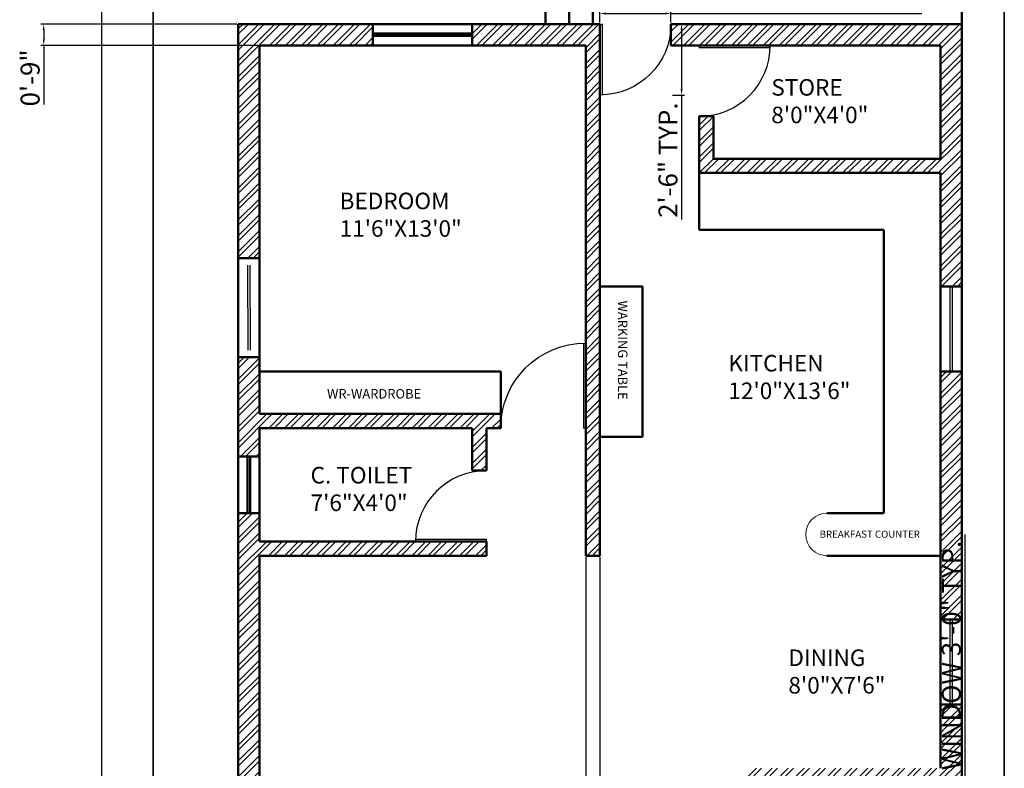
# Model space of a CAD drawing. Units: inches. Extents: x 1986 to 21484, y -1816 to 2016.
# Tile 47 of 85: x 3482 to 3899, y 1538 to 1855. Entities that reach past the tile are written whole.
import ezdxf

# ---------------------------------------------------------------- set-up
doc = ezdxf.new("R2010")
doc.units = ezdxf.units.IN
for name, color, linetype, lineweight in [('A-ANNO-DIMS', 2, 'Continuous', 18), ('A-ANNO-TEXT', 7, 'Continuous', 18), ('A-AREA-IDEN', 3, 'Continuous', 18), ('A-DOOR', 3, 'Continuous', 25), ('A-FURN', 8, 'Continuous', 18), ('A-GLAZ', 4, 'Continuous', 25), ('A-WALL', 7, 'Continuous', 50), ('A-WALL-PATT', 8, 'Continuous', 13), ('C-PROP', 7, 'Continuous', 35)]:
    doc.layers.add(name, color=color, linetype=linetype, lineweight=lineweight)
doc.styles.get("Standard").update_dxf_attribs({"font": 'arial.ttf'})
doc.dimstyles.new('ISO-25', dxfattribs={"dimtxt": 8, "dimasz": 2.5, "dimexe": 1.25, "dimexo": 0.625, "dimtad": 1, "dimdec": 1, "dimlunit": 3, "dimtxsty": 'Standard', "dimcen": 2.5, "dimadec": 0, "dimazin": 0, "dimtfac": 1, "dimtdec": 1, "dimtmove": 0, "dimatfit": 3, "dimfxl": 1, "dimarcsym": 0})

# ---------------------------------------------------------------- blocks, each defined once
blk = doc.blocks.new('*D32')
at = {"layer": 'A-ANNO-DIMS', "color": 0, "lineweight": -2, "transparency": 16777216}
for p, q in [((3538.28, 1900.75), (3515.81, 1900.75)), ((3517.06, 1898.25), (3517.06, 1069.25)), ((3538.28, 1066.75), (3515.81, 1066.75))]:
    blk.add_line(p, q, dxfattribs=at)
at = {"layer": 'A-ANNO-DIMS', "color": 0, "transparency": 16777216}
for points in [[(3516.64, 1898.25), (3517.47, 1898.25), (3517.06, 1900.75)], [(3516.64, 1069.25), (3517.47, 1069.25), (3517.06, 1066.75)]]:
    blk.add_solid(points, dxfattribs=at)
at = {"layer": 'Defpoints', "color": 0, "transparency": 16777216}
for p in [(3538.91, 1900.75), (3517.06, 1066.75), (3538.91, 1066.75)]:
    blk.add_point(p, dxfattribs=at)
at = {"layer": 'A-ANNO-DIMS', "color": 0, "transparency": 16777216, "insert": (3512.35, 1483.75), "char_height": 8, "attachment_point": 5, "rotation": 90}
blk.add_mtext('69\'-6"', dxfattribs=at)
blk = doc.blocks.new('D2')
for p, q in [((1722.5, 1505.46), (1722.5, 1475.46)), ((1723.5, 1505.46), (1723.5, 1475.46)), ((1722.5, 1475.46), (1723.5, 1475.46))]:
    blk.add_line(p, q)
blk.add_arc((1722.5, 1475.46), 30, 0, 90)
blk = doc.blocks.new('D1')
for p, q in [((1805.96, 1500.36), (1805.96, 1464.36)), ((1806.96, 1500.36), (1806.96, 1464.36)), ((1805.96, 1464.36), (1806.96, 1464.36))]:
    blk.add_line(p, q)
blk.add_arc((1805.96, 1464.36), 36, 0, 90)
blk = doc.blocks.new('WIN-36')
for p, q in [((0, 36), (0, 0)), ((0, 36), (0, 0)), ((1, 36), (1, 0))]:
    blk.add_line(p, q)
blk = doc.blocks.new('*D87')
at = {"layer": 'A-ANNO-DIMS', "color": 0, "lineweight": -2, "transparency": 16777216}
for p, q in [((3882.31, 1531.75), (3882.31, 1636.74)), ((3877.53, 1531.75), (3883.56, 1531.75)), ((3882.31, 1498.25), (3882.31, 1529.25)), ((3877.53, 1495.75), (3883.56, 1495.75))]:
    blk.add_line(p, q, dxfattribs=at)
at = {"layer": 'A-ANNO-DIMS', "color": 0, "transparency": 16777216}
for points in [[(3881.89, 1529.25), (3882.72, 1529.25), (3882.31, 1531.75)], [(3881.89, 1498.25), (3882.72, 1498.25), (3882.31, 1495.75)]]:
    blk.add_solid(points, dxfattribs=at)
at = {"layer": 'Defpoints', "color": 0, "transparency": 16777216}
for p in [(3876.91, 1531.75), (3882.31, 1531.75), (3876.91, 1495.75)]:
    blk.add_point(p, dxfattribs=at)
at = {"layer": 'A-ANNO-DIMS', "color": 0, "transparency": 16777216, "insert": (3877.54, 1585.49), "char_height": 8, "attachment_point": 5, "rotation": 90}
blk.add_mtext('WINDOW 3\'-0" TYP.', dxfattribs=at)
blk = doc.blocks.new('*D91')
at = {"layer": 'A-ANNO-DIMS', "color": 0, "lineweight": -2, "transparency": 16777216}
for p, q in [((3727.91, 1853.38), (3727.91, 1858.5)), ((3730.41, 1857.25), (3755.41, 1857.25)), ((3757.91, 1853.38), (3757.91, 1858.5)), ((3757.91, 1857.25), (3864.05, 1857.25))]:
    blk.add_line(p, q, dxfattribs=at)
at = {"layer": 'A-ANNO-DIMS', "color": 0, "transparency": 16777216}
for points in [[(3730.41, 1857.67), (3730.41, 1856.84), (3727.91, 1857.25)], [(3755.41, 1857.67), (3755.41, 1856.84), (3757.91, 1857.25)]]:
    blk.add_solid(points, dxfattribs=at)
at = {"layer": 'Defpoints', "color": 0, "transparency": 16777216}
for p in [(3757.91, 1857.25), (3727.91, 1852.75), (3757.91, 1852.75)]:
    blk.add_point(p, dxfattribs=at)
at = {"layer": 'A-ANNO-DIMS', "color": 0, "transparency": 16777216, "insert": (3812.23, 1862.02), "char_height": 8, "attachment_point": 5}
blk.add_mtext('DOOR D2 2\'-6" TYP.', dxfattribs=at)
blk = doc.blocks.new('*D92')
at = {"layer": 'A-ANNO-DIMS', "color": 0, "lineweight": -2, "transparency": 16777216}
for p, q in [((3758.53, 1852.75), (3763.66, 1852.75)), ((3762.41, 1850.25), (3762.41, 1825.25)), ((3758.53, 1822.75), (3763.66, 1822.75)), ((3762.41, 1822.75), (3762.41, 1770.1))]:
    blk.add_line(p, q, dxfattribs=at)
at = {"layer": 'A-ANNO-DIMS', "color": 0, "transparency": 16777216}
for points in [[(3761.99, 1850.25), (3762.82, 1850.25), (3762.41, 1852.75)], [(3761.99, 1825.25), (3762.82, 1825.25), (3762.41, 1822.75)]]:
    blk.add_solid(points, dxfattribs=at)
at = {"layer": 'Defpoints', "color": 0, "transparency": 16777216}
for p in [(3757.91, 1852.75), (3757.91, 1822.75), (3762.41, 1822.75)]:
    blk.add_point(p, dxfattribs=at)
at = {"layer": 'A-ANNO-DIMS', "color": 0, "transparency": 16777216, "insert": (3757.7, 1795.18), "char_height": 8, "attachment_point": 5, "rotation": 90}
blk.add_mtext('2\'-6" TYP.', dxfattribs=at)
blk = doc.blocks.new('*D96')
at = {"layer": 'A-ANNO-DIMS', "color": 0, "lineweight": -2, "transparency": 16777216}
for p, q in [((3539.82, 1864.46), (3539.82, 1858.21)), ((3577.11, 1864.46), (3577.11, 1858.21)), ((3542.32, 1859.46), (3574.61, 1859.46)), ((3577.11, 1859.46), (3648.26, 1859.46))]:
    blk.add_line(p, q, dxfattribs=at)
at = {"layer": 'A-ANNO-DIMS', "color": 0, "transparency": 16777216}
for points in [[(3542.32, 1859.88), (3542.32, 1859.05), (3539.82, 1859.46)], [(3574.61, 1859.88), (3574.61, 1859.05), (3577.11, 1859.46)]]:
    blk.add_solid(points, dxfattribs=at)
at = {"layer": 'Defpoints', "color": 0, "transparency": 16777216}
for p in [(3539.82, 1865.09), (3577.11, 1865.09), (3577.11, 1859.46)]:
    blk.add_point(p, dxfattribs=at)
at = {"layer": 'A-ANNO-DIMS', "color": 0, "transparency": 16777216, "insert": (3613.94, 1864.23), "char_height": 8, "attachment_point": 5}
blk.add_mtext('3\'-1 1/2" TYP.', dxfattribs=at)
blk = doc.blocks.new('*D127')
at = {"layer": 'A-ANNO-DIMS', "color": 0, "lineweight": -2, "transparency": 16777216}
for p, q in [((3574.28, 1852.75), (3491.41, 1852.75)), ((3492.66, 1850.25), (3492.66, 1846.25)), ((3583.28, 1843.75), (3491.41, 1843.75)), ((3492.66, 1843.75), (3492.66, 1818.74))]:
    blk.add_line(p, q, dxfattribs=at)
at = {"layer": 'A-ANNO-DIMS', "color": 0, "transparency": 16777216}
for points in [[(3492.24, 1850.25), (3493.07, 1850.25), (3492.66, 1852.75)], [(3492.24, 1846.25), (3493.07, 1846.25), (3492.66, 1843.75)]]:
    blk.add_solid(points, dxfattribs=at)
at = {"layer": 'Defpoints', "color": 0, "transparency": 16777216}
for p in [(3574.91, 1852.75), (3492.66, 1843.75), (3583.91, 1843.75)]:
    blk.add_point(p, dxfattribs=at)
at = {"layer": 'A-ANNO-DIMS', "color": 0, "transparency": 16777216, "insert": (3487.95, 1829.99), "char_height": 8, "attachment_point": 5, "rotation": 90}
blk.add_mtext('0\'-9"', dxfattribs=at)
blk = doc.blocks.new('*D128')
at = {"layer": 'A-ANNO-DIMS', "color": 0, "lineweight": -2, "transparency": 16777216}
for p, q in [((3721.91, 1627.13), (3721.91, 953.11)), ((3727.91, 1627.13), (3727.91, 953.11)), ((3719.41, 954.36), (3716.91, 954.36)), ((3721.91, 954.36), (3727.91, 954.36)), ((3730.41, 954.36), (3755.42, 954.36))]:
    blk.add_line(p, q, dxfattribs=at)
at = {"layer": 'A-ANNO-DIMS', "color": 0, "transparency": 16777216}
for points in [[(3719.41, 954.78), (3719.41, 953.95), (3721.91, 954.36)], [(3730.41, 954.78), (3730.41, 953.95), (3727.91, 954.36)]]:
    blk.add_solid(points, dxfattribs=at)
at = {"layer": 'Defpoints', "color": 0, "transparency": 16777216}
for p in [(3721.91, 1627.75), (3727.91, 1627.75), (3727.91, 954.36)]:
    blk.add_point(p, dxfattribs=at)
at = {"layer": 'A-ANNO-DIMS', "color": 0, "transparency": 16777216, "insert": (3744.17, 959.07), "char_height": 8, "attachment_point": 5}
blk.add_mtext('0\'-6"', dxfattribs=at)

msp = doc.modelspace()

# ---------------------------------------------------------------- hatches: boundary and pattern name
at = {"layer": 'A-WALL-PATT'}
h = msp.add_hatch(dxfattribs=at)
h.set_pattern_fill('ANSI32', color=256, scale=0.5)
h.paths.add_polyline_path([(3631.91, 1852.75), (3574.91, 1852.75), (3574.91, 1753.75), (3583.91, 1753.75), (3583.91, 1843.75), (3631.91, 1843.75)])
h.paths.add_polyline_path([(3727.91, 1852.75), (3673.91, 1852.75), (3673.91, 1843.75), (3721.91, 1843.75), (3721.91, 1627.75), (3727.91, 1627.75)])
h.paths.add_polyline_path([(3880.91, 1852.75), (3757.91, 1852.75), (3757.91, 1843.75), (3871.91, 1843.75), (3871.91, 1795.75), (3775.91, 1795.75), (3775.91, 1813.75), (3769.91, 1813.75), (3769.91, 1789.75), (3871.91, 1789.75), (3871.91, 1741.75), (3880.91, 1741.75)])
h.paths.add_polyline_path([(3880.91, 1705.75), (3871.91, 1705.75), (3871.91, 1600.75), (3880.91, 1600.75)])
h.paths.add_polyline_path([(3685.91, 1687.75), (3583.91, 1687.75), (3583.91, 1711.75), (3574.91, 1711.75), (3574.91, 1669.75), (3583.91, 1669.75), (3583.91, 1681.75), (3673.91, 1681.75), (3673.91, 1663.75), (3679.91, 1663.75), (3679.91, 1681.75), (3685.91, 1681.75)])
h.paths.add_polyline_path([(3583.91, 1399.75), (3574.91, 1399.75), (3574.91, 1276.75), (3583.91, 1276.75)])
h.paths.add_polyline_path([(3648.41, 1387.75), (3631.91, 1387.75), (3631.91, 1378.75), (3648.41, 1378.75)])
h.paths.add_polyline_path([(3715.91, 1387.75), (3690.41, 1387.75), (3690.41, 1378.75), (3706.91, 1378.75), (3706.91, 1189.75), (3715.91, 1189.75)])
h.paths.add_polyline_path([(3880.91, 1387.75), (3871.91, 1387.75), (3751.91, 1387.75), (3751.91, 1381.75), (3871.91, 1381.75), (3871.91, 1363.75), (3880.91, 1363.75)])
h.paths.add_polyline_path([(3880.91, 1441.75), (3871.91, 1441.75), (3871.91, 1423.75), (3880.91, 1423.75)])
h.paths.add_polyline_path([(3880.91, 1495.75), (3871.91, 1495.75), (3871.91, 1477.75), (3880.91, 1477.75)])
h.paths.add_polyline_path([(3880.91, 1339.75), (3871.91, 1339.75), (3871.91, 1321.75), (3775.91, 1321.75), (3775.91, 1351.75), (3769.91, 1351.75), (3769.91, 1315.75), (3871.91, 1315.75), (3871.91, 1303.75), (3880.91, 1303.75)])
h.paths.add_polyline_path([(3880.91, 1261.75), (3871.91, 1261.75), (3871.91, 1189.75), (3880.91, 1189.75)])
h.paths.add_polyline_path([(3880.91, 1147.75), (3871.91, 1147.75), (3871.91, 1123.75), (3763.91, 1123.75), (3763.91, 1114.75), (3880.91, 1114.75)])
h.paths.add_polyline_path([(3721.91, 1123.75), (3715.91, 1123.75), (3715.91, 1147.75), (3706.91, 1147.75), (3706.91, 1114.75), (3721.91, 1114.75)])
h.paths.add_polyline_path([(3880.91, 1564.75), (3871.91, 1564.75), (3871.91, 1537.75), (3789.91, 1537.75), (3789.91, 1531.75), (3871.91, 1531.75), (3880.91, 1531.75)])
h.paths.add_polyline_path([(3583.91, 1627.75), (3679.91, 1627.75), (3679.91, 1633.75), (3649.91, 1633.75), (3583.91, 1633.75), (3583.91, 1645.75), (3574.91, 1645.75), (3574.91, 1441.75), (3583.91, 1441.75)])
h.paths.add_polyline_path([(3733.26, 1736.83), (3733.26, 1685.78), (3741.8, 1685.78), (3741.8, 1736.83)], flags=9)
h.paths.add_polyline_path([(3763.81, 1864.73), (3812.77, 1864.73), (3812.77, 1891.35), (3763.81, 1891.35)], flags=9)
h.paths.add_polyline_path([(3797.97, 1806.84), (3841.79, 1806.84), (3841.79, 1833.45), (3797.97, 1833.45)], flags=25)
h.paths.add_polyline_path([(3779.25, 1690.08), (3833.38, 1690.08), (3833.38, 1716.69), (3779.25, 1716.69)], flags=9)
h.paths.add_polyline_path([(3805.23, 1565.41), (3849.03, 1565.41), (3849.03, 1592.03), (3805.23, 1592.03)], flags=9)
h.paths.add_polyline_path([(3638.57, 1496.24), (3711.25, 1496.24), (3711.25, 1522.85), (3638.57, 1522.85)], flags=9)
h.paths.add_polyline_path([(3617.97, 1320.51), (3666.93, 1320.51), (3666.93, 1347.12), (3617.97, 1347.12)], flags=9)
h.paths.add_polyline_path([(3768.51, 1208.98), (3836.51, 1208.98), (3836.51, 1235.59), (3768.51, 1235.59)], flags=9)
h.paths.add_polyline_path([(3791.7, 1338.54), (3844.53, 1338.54), (3844.53, 1365.15), (3791.7, 1365.15)], flags=9)
h.paths.add_polyline_path([(3614.85, 1758.76), (3671.08, 1758.76), (3671.08, 1785.38), (3614.85, 1785.38)], flags=9)
h.paths.add_polyline_path([(3603.38, 1642.68), (3655.11, 1642.68), (3655.11, 1669.29), (3603.38, 1669.29)], flags=9)

# ---------------------------------------------------------------- linework, layer by layer
at = {"layer": 'A-FURN'}
msp.add_arc((3823.91, 1636.75), 9, 90, 270, dxfattribs=at)
at = {"layer": 'A-WALL'}
for p, q in [((3704.91, 1900.75), (3704.91, 1852.75)), ((3714.91, 1900.75), (3714.91, 1852.75)), ((3724.91, 1900.75), (3724.91, 1852.75)), ((3880.91, 1900.75), (3880.91, 1114.75)), ((3574.91, 1852.75), (3727.91, 1852.75)), ((3574.91, 1276.75), (3574.91, 1852.75)), ((3631.91, 1843.75), (3631.91, 1852.75)), ((3673.91, 1843.75), (3673.91, 1852.75)), ((3727.91, 1627.75), (3727.91, 1852.75)), ((3757.91, 1852.75), (3880.91, 1852.75)), ((3757.91, 1843.75), (3757.91, 1852.75)), ((3631.91, 1848.75), (3673.91, 1848.75)), ((3631.91, 1847.75), (3673.91, 1847.75)), ((3583.91, 1843.75), (3721.91, 1843.75)), ((3583.91, 1687.75), (3583.91, 1843.75)), ((3721.91, 1627.75), (3721.91, 1843.75)), ((3757.91, 1843.75), (3871.91, 1843.75)), ((3871.91, 1843.75), (3871.91, 1795.75)), ((3769.91, 1813.75), (3775.91, 1813.75)), ((3769.91, 1813.75), (3769.91, 1765.75)), ((3775.91, 1813.75), (3775.91, 1795.75)), ((3775.91, 1795.75), (3871.91, 1795.75)), ((3769.91, 1789.75), (3871.91, 1789.75)), ((3871.91, 1789.75), (3871.91, 1537.75)), ((3769.91, 1765.75), (3847.91, 1765.75)), ((3847.91, 1765.75), (3847.91, 1645.75)), ((3574.91, 1753.75), (3583.91, 1753.75)), ((3727.91, 1741.75), (3745.91, 1741.75)), ((3745.91, 1678.13), (3745.91, 1741.75)), ((3871.91, 1741.75), (3880.91, 1741.75)), ((3574.91, 1711.75), (3583.91, 1711.75)), ((3583.91, 1705.75), (3685.91, 1705.75)), ((3685.91, 1681.75), (3685.91, 1705.75)), ((3871.91, 1705.75), (3880.91, 1705.75)), ((3583.91, 1687.75), (3685.91, 1687.75)), ((3583.91, 1681.75), (3673.91, 1681.75)), ((3583.91, 1633.75), (3583.91, 1681.75)), ((3673.91, 1663.75), (3673.91, 1681.75)), ((3679.91, 1681.75), (3685.91, 1681.75)), ((3679.91, 1663.75), (3679.91, 1681.75)), ((3727.91, 1678.13), (3745.91, 1678.13)), ((3574.91, 1669.75), (3583.91, 1669.75)), ((3578.91, 1645.75), (3578.91, 1669.75)), ((3579.91, 1645.75), (3579.91, 1669.75)), ((3673.91, 1663.75), (3679.91, 1663.75)), ((3574.91, 1645.75), (3583.91, 1645.75)), ((3823.91, 1645.75), (3847.91, 1645.75)), ((3583.91, 1633.75), (3679.91, 1633.75)), ((3679.91, 1627.75), (3679.91, 1633.75)), ((3583.91, 1276.75), (3583.91, 1627.75)), ((3583.91, 1627.75), (3679.91, 1627.75)), ((3721.91, 1627.75), (3727.91, 1627.75)), ((3823.91, 1627.75), (3871.91, 1627.75)), ((3871.91, 1600.75), (3880.91, 1600.75)), ((3871.91, 1564.75), (3880.91, 1564.75))]:
    msp.add_line(p, q, dxfattribs=at)
at = {"layer": 'C-PROP'}
msp.add_lwpolyline([(3538.91, 1900.75), (3898.91, 1900.75), (3898.91, 1066.75), (3538.91, 1066.75)], close=True, dxfattribs=at)

# ---------------------------------------------------------------- block references
at = {"layer": 'A-DOOR', "xscale": -1, "rotation": 180}
msp.add_blockref('D2', (2005.41, 3328.21), dxfattribs=at)
at = {"layer": 'A-DOOR'}
for p, rotation in [((2294.45, 3566.25), 270), ((5155.36, -88.75), 90)]:
    msp.add_blockref('D2', p, dxfattribs=dict(at, rotation=rotation))
at = {"layer": 'A-DOOR', "xscale": -1}
msp.add_blockref('D1', (5527.87, 217.39), dxfattribs=at)
at = {"layer": 'A-GLAZ', "rotation": 0.302793432207276}
msp.add_blockref('WIN-36', (3579, 1714.75), dxfattribs=at)
at = {"layer": 'A-GLAZ'}
for p in [(3875.91, 1705.75), (3875.91, 1564.75)]:
    msp.add_blockref('WIN-36', p, dxfattribs=at)

# ---------------------------------------------------------------- texts
at = {"layer": 'A-ANNO-TEXT', "insert": (3739.54, 1735.75), "char_height": 4, "attachment_point": 1, "rotation": 270}
msp.add_mtext_dynamic_manual_height_columns('{\\fTimes New Roman|b0|i0|c0|p18;WARKING TABLE}', width=105.6127, gutter_width=12.5, heights=[0], dxfattribs=at)
at = {"layer": 'A-ANNO-TEXT', "attachment_point": 1}
for s, insert, char_height in [('{\\fTimes New Roman|b0|i0|c0|p18;WR-WARDROBE}', (3612.48, 1698.29), 4), ('{\\fTimes New Roman|b0|i0|c0|p18;BREAKFAST COUNTER}', (3820.8, 1638.37), 3)]:
    msp.add_mtext_dynamic_manual_height_columns(s, width=105.6127, gutter_width=12.5, heights=[0], dxfattribs=dict(at, insert=insert, char_height=char_height))
at = {"layer": 'A-AREA-IDEN', "char_height": 7, "attachment_point": 1}
for s, insert in [('{\\fTimes New Roman|b0|i0|c0|p18;STORE\\P8\'0"X4\'0"}', (3800.37, 1829.49)), ('{\\fTimes New Roman|b0|i0|c0|p18;BEDROOM \\P11\'6"X13\'0"}', (3617.81, 1781.42)), ('{\\fTimes New Roman|b0|i0|c0|p18;KITCHEN\\P12\'0"X13\'6"}', (3782.21, 1712.73)), ('{\\fTimes New Roman|b0|i0|c0|p18;C. TOILET\\P7\'6"X4\'0"}', (3605.51, 1665.33)), ('{\\fTimes New Roman|b0|i0|c0|p18;DINING\\P8\'0"X7\'6"}', (3807.6, 1588.07))]:
    msp.add_mtext_dynamic_manual_height_columns(s, width=105.6127, gutter_width=12.5, heights=[0], dxfattribs=dict(at, insert=insert))

# ---------------------------------------------------------------- dimensions: what is measured, and where the dimension line sits
at = {"layer": 'A-ANNO-DIMS'}
for base, p1, p2, override, picture, middle in [((3517.06, 1066.75), (3538.91, 1900.75), (3538.91, 1066.75), {"dimclrd": 0, "dimclre": 0, "dimclrt": 0}, '*D32', (3512.35, 1483.75)), ((3492.66, 1843.75), (3574.91, 1852.75), (3583.91, 1843.75), {"dimdec": 1, "dimlfac": 1, "dimrnd": 0, "dimzin": 1, "dimdsep": 46, "dimlunit": 4, "dimfrac": 2}, '*D127', (3487.95, 1829.99))]:
    dim = msp.add_linear_dim(base=base, p1=p1, p2=p2, angle=90, dimstyle='ISO-25', override=override, dxfattribs=at)
    dim.commit()
    dim.dimension.update_dxf_attribs({"geometry": picture, "text_midpoint": middle})
for base, p1, p2, text, picture, middle in [((3757.91, 1857.25), (3727.91, 1852.75), (3757.91, 1852.75), 'DOOR D2 <> TYP.', '*D91', (3812.23, 1862.02)), ((3577.11, 1859.46), (3539.82, 1865.09), (3577.11, 1865.09), '<> TYP.', '*D96', (3613.94, 1864.23))]:
    dim = msp.add_linear_dim(base=base, p1=p1, p2=p2, text=text, dimstyle='ISO-25', override={"dimdec": 1, "dimrnd": 0, "dimzin": 1, "dimlunit": 4, "dimfrac": 2}, dxfattribs=at)
    dim.commit()
    dim.dimension.update_dxf_attribs({"geometry": picture, "text_midpoint": middle})
for base, p1, p2, angle, text, picture, middle in [((3762.41, 1822.75), (3757.91, 1852.75), (3757.91, 1822.75), 270, '<> TYP.', '*D92', (3757.7, 1795.18)), ((3882.31, 1531.75), (3876.91, 1495.75), (3876.91, 1531.75), 90, 'WINDOW <> TYP.', '*D87', (3877.54, 1585.49))]:
    dim = msp.add_linear_dim(base=base, p1=p1, p2=p2, angle=angle, text=text, dimstyle='ISO-25', override={"dimdec": 1, "dimrnd": 0, "dimzin": 1, "dimlunit": 4, "dimfrac": 2}, dxfattribs=at)
    dim.commit()
    dim.dimension.update_dxf_attribs({"geometry": picture, "text_midpoint": middle})
dim = msp.add_linear_dim(base=(3727.91, 954.36), p1=(3721.91, 1627.75), p2=(3727.91, 1627.75), dimstyle='ISO-25', override={"dimdec": 1, "dimlfac": 1, "dimrnd": 0, "dimzin": 1, "dimdsep": 46, "dimlunit": 4, "dimfrac": 2}, dxfattribs=at)
dim.commit()
dim.dimension.update_dxf_attribs({"geometry": '*D128', "text_midpoint": (3744.17, 959.07)})

doc.saveas('drawing.dxf')
